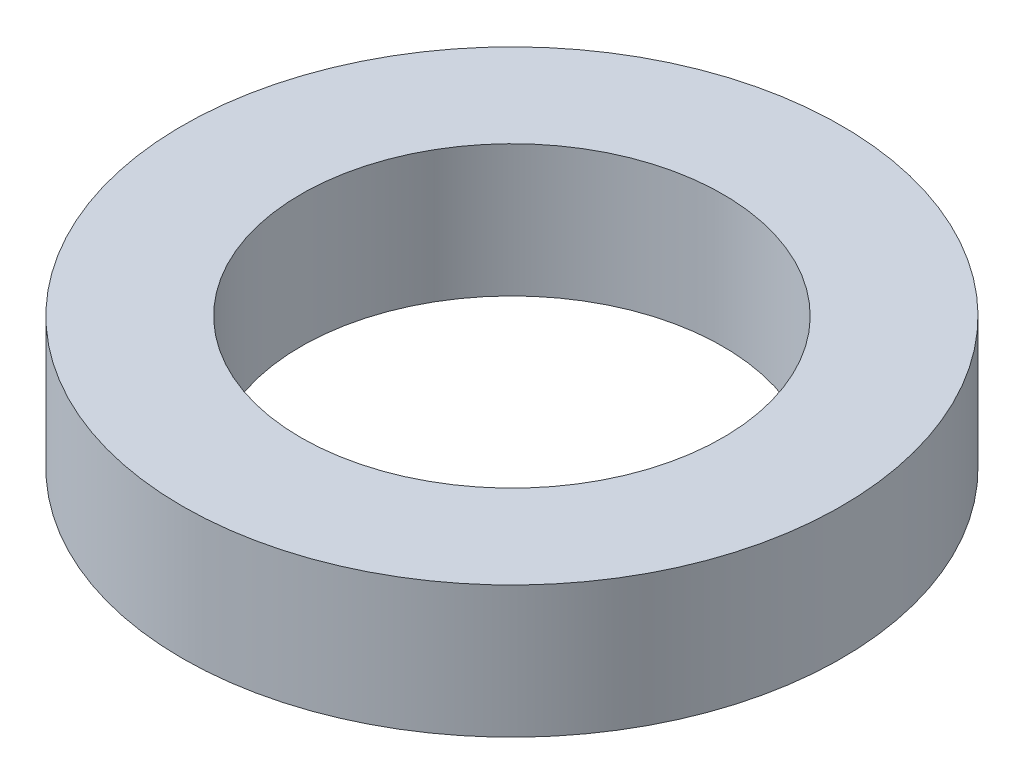
SolidWorks part; units mm, degrees
material "Plain Carbon Steel"
ref_plane "Front Plane" through (0, 0, 0) normal (0, 0, 1) x (1, 0, 0)
ref_plane "Top Plane" through (0, 0, 0) normal (0, 1, 0) x (1, 0, 0)
ref_plane "Right Plane" through (0, 0, 0) normal (1, 0, 0) x (0, 0, -1)
sketch "Washer Profile Ø50-Ø32" plane through (0, 0, 0) normal (0, 1, 0) x (1, 0, 0)
  circle A0 centre (0, 0) radius 25
  circle A1 centre (0, 0) radius 16
  dimension "D1" = 50
  dimension "D2" = 32
extrude "Washer Body 10mm" add sketch "Washer Profile Ø50-Ø32" along normal blind 10
